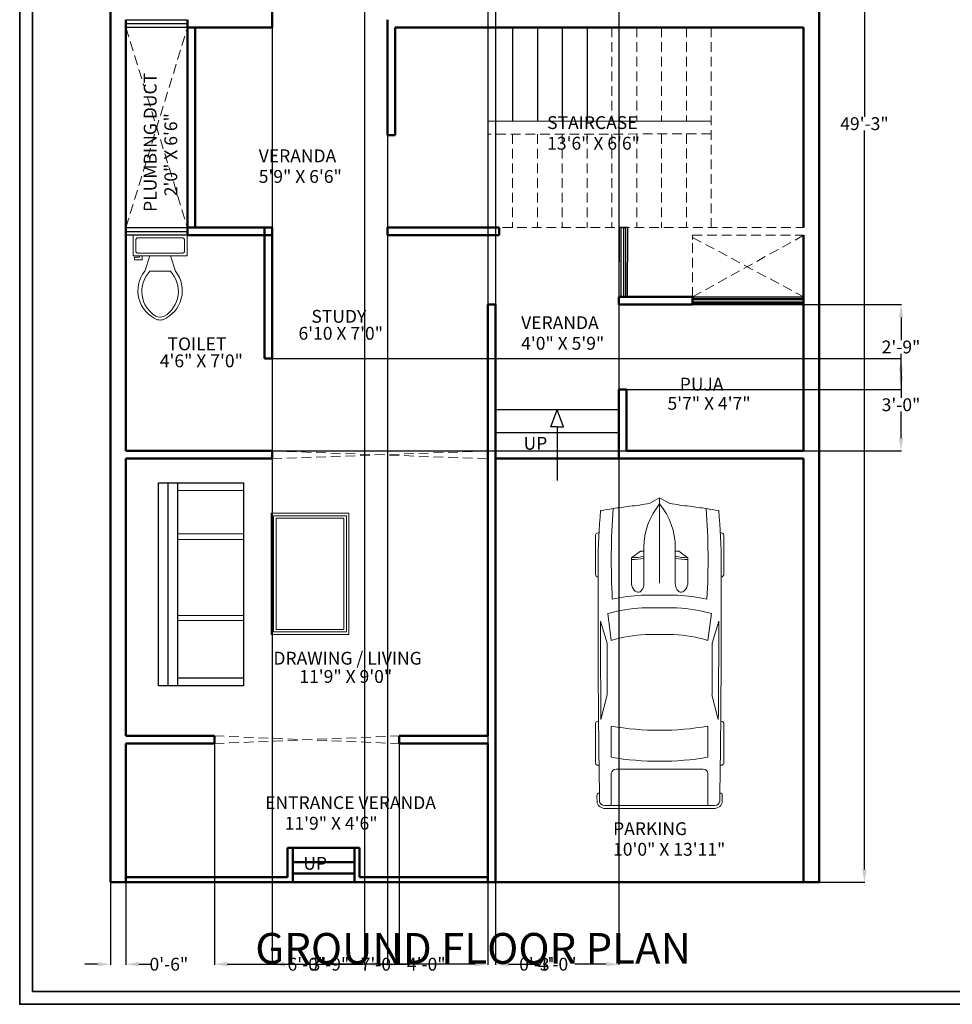
# Model space of a CAD drawing. Units: inches. Extents: x 396 to 1141, y -378 to 313.
# Tile 1 of 3: x 400 to 764, y -378 to 6. Entities that reach past the tile are written whole.
import ezdxf

# ---------------------------------------------------------------- set-up
doc = ezdxf.new("R2010")
doc.units = ezdxf.units.IN
doc.header["$MEASUREMENT"] = 0
doc.linetypes.add('DASHED', pattern=[19.05, 12.7, -6.35])
for name, color, linetype, lineweight in [('A-ANNO-DIMS', 2, 'Continuous', 18), ('A-ANNO-TTLB', 7, 'Continuous', 35), ('A-AREA-IDEN', 3, 'Continuous', 25), ('A-EQPM', 8, 'Continuous', 13), ('A-FLOR-FIXT', 150, 'Continuous', 18), ('A-FLOR-OVHD', 8, 'DASHED', 18), ('A-FLOR-STRS', 220, 'Continuous', 25), ('A-FLOR-STRS-OVHD', 220, 'DASHED', 18), ('A-FURN', 30, 'Continuous', 18), ('A-GLAZ', 4, 'Continuous', 25), ('A-WALL', 7, 'Continuous', 50)]:
    doc.layers.add(name, color=color, linetype=linetype, lineweight=lineweight)
doc.styles.get("Standard").update_dxf_attribs({"font": 'arial.ttf'})
doc.dimstyles.get("Standard").update_dxf_attribs({"dimtxt": 5, "dimasz": 5, "dimexe": 0.18, "dimexo": 0.0625, "dimgap": 0.09, "dimtad": 0, "dimtih": 1, "dimtoh": 1, "dimdec": 1, "dimzin": 0, "dimdsep": 46, "dimlunit": 4, "dimtxsty": 'Standard', "dimcen": 0.09, "dimadec": 0, "dimazin": 0, "dimtfac": 1, "dimtdec": 1, "dimtofl": 0, "dimtmove": 0, "dimatfit": 3, "dimfxl": 1, "dimtolj": 1, "dimtzin": 0, "dimarcsym": 0})

# ---------------------------------------------------------------- blocks, each defined once
blk = doc.blocks.new('*U6')
for p, q in [((9.5, -6), (9.5, -2)), ((-10, -8.5), (-8, -8.5)), ((-10, -9.5), (-10, -8.5)), ((-7, -9.5), (-10, -9.5)), ((-8, -8.5), (-8, -8)), ((-7, -8), (-7, -9.5)), ((-4, -8), (-6, -14)), ((4, -8), (6, -14)), ((4, -14), (-4, -14))]:
    blk.add_line(p, q)
blk.add_lwpolyline([(10.5, -8), (10.5, 0), (-10.5, 0), (-10.5, -8)], close=True)
for points in [[(-9.5, -2), (-9.5, -6)], [(8.5, -1), (-8.5, -1)], [(-8.5, -7), (8.5, -7)]]:
    blk.add_lwpolyline(points)
for centre, radius, start, end in [((-8.62, -1.88), 0.884, 81.8699, 188.1301), ((8.62, -1.88), 0.884, 351.8699, 98.1301), ((-8.62, -6.12), 0.884, 171.8699, 278.1301), ((8.62, -6.12), 0.884, 261.8699, 8.1301), ((3.52, -21.58), 12.17, 141.4691, 247.9714), ((4.2, -21.82), 11.33, 136.3677, 238.9468), ((-3.52, -21.58), 12.17, 292.0284, 38.5307), ((-4.2, -21.82), 11.33, 301.053, 43.6321), ((0, -27.88), 4, 245.7318, 294.2682), ((0, -29), 4, 254.8605, 285.1395)]:
    blk.add_arc(centre, radius, start, end)
blk = doc.blocks.new('*U8')
for p, q in [((21.1, 37.41), (21.1, 36.83)), ((46.55, 38.89), (22.35, 38.89)), ((47.8, 37.39), (47.8, 37.41)), ((87.99, 31.87), (74.76, 35.92)), ((135.45, 37.07), (135.45, 37.41)), ((136.7, 38.89), (160.9, 38.89)), ((162.15, 37.41), (162.15, 36.77)), ((70.03, 31.54), (86.41, 29.35)), ((134.31, 35.6), (119.29, 31.78)), ((186.47, -33.5), (186.47, 33.5)), ((188.4, -32.76), (188.4, 32.76)), ((138.42, 29.35), (157.25, 29.35)), ((164.52, 26.39), (164.52, -26.39)), ((186.47, 29.35), (167.01, 29.35)), ((32.27, 11.63), (36.13, 17.17)), ((36.13, 17.17), (50.94, 17.17)), ((3.27, 6.13), (0.1, 0.41)), ((29.77, 9.51), (51.68, 9.51)), ((32.12, 9.51), (32.12, 11.15)), ((58.92, -10.77), (58.92, 10.77)), ((66.55, -10.53), (66.55, 10.53)), ((82.74, 8.5), (82.74, -8.5)), ((186.47, -10.53), (186.47, 10.53)), ((0, 0), (51.68, 0)), ((0.1, -0.41), (3.27, -6.13)), ((29.77, -9.51), (51.68, -9.51)), ((32.12, -9.51), (32.12, -11.15)), ((32.27, -11.63), (36.13, -17.17)), ((36.13, -17.17), (50.94, -17.17)), ((86.41, -29.35), (70.03, -31.54)), ((157.25, -29.35), (138.42, -29.35)), ((167.01, -29.35), (186.47, -29.35)), ((87.99, -31.87), (74.76, -35.92)), ((134.31, -35.6), (119.29, -31.78)), ((21.1, -37.41), (21.1, -36.83)), ((46.55, -38.89), (22.35, -38.89)), ((47.8, -37.39), (47.8, -37.41)), ((135.45, -37.07), (135.45, -37.41)), ((136.7, -38.89), (160.9, -38.89)), ((162.15, -37.41), (162.15, -36.77))]:
    blk.add_line(p, q)
for centre, major_axis, ratio, start_param, end_param in [((266.03, -27.52), (0, 313.31), 0.842304, 1.367076, 1.39176), ((41.19, -490.86), (0, 528.23), 0.842304, 0.00281, 0.075598), ((22.35, 37.41), (0, -1.48), 0.842304, 3.141593, 4.712389), ((64.48, -10555.62), (0, 10593.03), 0.842304, -0.013397, 0.002797), ((46.55, 37.41), (0, 1.48), 0.842304, -1.570796, 0), ((64.48, -10555.62), (0, -10591.55), 0.842304, 3.133765, 3.140441), ((136.7, 37.41), (0, -1.48), 0.842304, 3.141593, 4.712389), ((160.9, 37.41), (0, 1.48), 0.842304, -1.570796, 0), ((180.63, 35.84), (0, 2.22), 0.842304, -0.013017, 1.249894), ((64.48, -10556.36), (0, 10595.31), 0.842304, -0.013397, -0.013017), ((183.98, 33.5), (0, -2.96), 0.842304, 1.570796, 3.128196), ((183.98, 32.76), (0, -5.25), 0.842304, 1.570796, 3.128196), ((135.29, 5.39), (0, 81.77), 0.842304, 1.245306, 1.50788), ((95.79, -3666.35), (0, -3698.24), 0.842304, 3.134049, 3.144098), ((259.18, -27.52), (0, -305.3), 0.842304, 4.528606, 4.561838), ((37.47, -593.96), (0, -623.33), 0.842304, 3.096046, 3.200911), ((134.4, 5.39), (0, -89.78), 0.842304, 4.449482, 4.652344), ((149.6, 2.8), (0, -79.58), 0.842304, 4.372215, 4.640744), ((17.08, 0), (0, 147.02), 0.842304, 4.511394, 4.913384), ((35.91, 0), (0, 147.02), 0.842304, 4.511394, 4.913384), ((167.01, 26.39), (0, 2.96), 0.842304, 0, 1.570796), ((-204.49, 52.4), (0, -250.96), 0.842304, 1.385369, 1.434372), ((13.04, 17.01), (0, 27.42), 0.842304, 4.435146, 4.718221), ((14.2, 17.01), (0, 27.42), 0.842304, 4.435146, 4.718221), ((50.79, 13.34), (6.34, -0.36), 0.603834, -1.395552, 1.581315), ((29.77, -46.66), (0, 56.17), 0.842304, 0, 0.590319), ((32.75, 11.15), (0, 0.74), 0.842304, 0.879714, 1.570796), ((0.62, 0), (0, -0.74), 0.842304, 4.131459, 5.293319), ((29.77, 46.66), (0, 56.17), 0.842304, 2.551274, 3.141593), ((-204.49, -52.4), (0, 250.96), 0.842304, -1.434372, -1.385369), ((32.75, -11.15), (0, -0.74), 0.842304, 4.712389, 5.403472), ((13.04, -17.01), (0, -27.42), 0.842304, 1.564964, 1.848039), ((14.2, -17.01), (0, -27.42), 0.842304, 1.564964, 1.848039), ((134.4, -5.39), (0, -89.78), 0.842304, -1.510751, -1.307889), ((135.29, -5.39), (0, -81.77), 0.842304, -1.50788, -1.245306), ((149.6, -2.8), (0, -79.58), 0.842304, -1.499151, -1.230623), ((259.18, 27.52), (0, 305.3), 0.842304, 1.721348, 1.754579), ((266.03, 27.52), (0, 313.31), 0.842304, 1.749832, 1.774517), ((37.47, 593.96), (0, -623.33), 0.842304, -0.059319, 0.045547), ((167.01, -26.39), (0, -2.96), 0.842304, 4.712389, 6.283185), ((64.48, 10555.62), (0, -10591.55), 0.842304, 0.001152, 0.007828), ((95.79, 3666.35), (0, -3698.24), 0.842304, -0.002505, 0.007544), ((183.98, -33.5), (0, 2.96), 0.842304, 3.15499, 4.712389), ((183.98, -32.76), (0, -5.25), 0.842304, 0.013397, 1.570796), ((41.19, 490.86), (0, -528.23), 0.842304, -0.075598, -0.00281), ((22.35, -37.41), (0, 1.48), 0.842304, 1.570796, 3.141593), ((64.48, 10555.62), (0, 10593.03), 0.842304, 3.138796, 3.15499), ((46.55, -37.41), (0, -1.48), 0.842304, 0, 1.570796), ((136.7, -37.41), (0, -1.48), 0.842304, -1.570796, 0), ((160.9, -37.41), (0, 1.48), 0.842304, 3.141593, 4.712389), ((180.63, -35.84), (0, -2.22), 0.842304, -1.249894, 0.013017), ((64.48, 10556.36), (0, 10595.31), 0.842304, 3.15461, 3.15499)]:
    blk.add_ellipse(centre, major_axis=major_axis, ratio=ratio, start_param=start_param, end_param=end_param)
at = {"extrusion": (0, 0, -1)}
blk.add_ellipse((50.79, -13.34), major_axis=(6.34, 0.36), ratio=0.603834, start_param=-1.395552, end_param=1.581315, dxfattribs=at)
blk = doc.blocks.new('*D10')
at = {"layer": 'A-ANNO-DIMS', "color": 0, "lineweight": -2, "ltscale": 0.3, "transparency": 16777216}
for p, q in [((711.68, 260.95), (729.49, 260.95)), ((729.31, 255.95), (729.31, -31.9)), ((729.31, -325.05), (729.31, -37.19)), ((711.68, -330.05), (729.49, -330.05))]:
    blk.add_line(p, q, dxfattribs=at)
at = {"layer": 'A-ANNO-DIMS', "color": 0, "ltscale": 0.3, "transparency": 16777216}
for points in [[(728.47, 255.95), (730.14, 255.95), (729.31, 260.95)], [(728.47, -325.05), (730.14, -325.05), (729.31, -330.05)]]:
    blk.add_solid(points, dxfattribs=at)
at = {"layer": 'Defpoints', "color": 0, "ltscale": 0.3, "transparency": 16777216}
for p in [(711.61, 260.95), (711.61, -330.05), (729.31, -330.05)]:
    blk.add_point(p, dxfattribs=at)
at = {"layer": 'A-ANNO-DIMS', "color": 0, "ltscale": 0.3, "transparency": 16777216, "insert": (729.31, -34.55), "char_height": 5, "attachment_point": 5}
blk.add_mtext('\\A1;49\'-3"', dxfattribs=at)
blk = doc.blocks.new('WIN-DUCT-700')
at = {"ltscale": 0.3}
blk.add_line((441.61, 4.45), (465.61, 4.45), dxfattribs=at)
blk.add_lwpolyline([(441.61, 5.95), (465.61, 5.95), (465.61, 2.95), (441.61, 2.95)], close=True, dxfattribs=at)
blk = doc.blocks.new('*D31')
at = {"layer": 'A-ANNO-DIMS', "color": 0, "lineweight": -2, "ltscale": 0.3, "transparency": 16777216}
for p, q in [((441.61, -328.11), (441.61, -362.18)), ((435.61, -330.11), (435.61, -362.18)), ((430.61, -362), (425.61, -362)), ((446.61, -362), (451.61, -362))]:
    blk.add_line(p, q, dxfattribs=at)
at = {"layer": 'A-ANNO-DIMS', "color": 0, "ltscale": 0.3, "transparency": 16777216}
for points in [[(430.61, -361.16), (430.61, -362.83), (435.61, -362)], [(446.61, -361.16), (446.61, -362.83), (441.61, -362)]]:
    blk.add_solid(points, dxfattribs=at)
at = {"layer": 'Defpoints', "color": 0, "ltscale": 0.3, "transparency": 16777216}
for p in [(441.61, -328.05), (435.61, -330.05), (441.61, -362)]:
    blk.add_point(p, dxfattribs=at)
at = {"layer": 'A-ANNO-DIMS', "color": 0, "ltscale": 0.3, "transparency": 16777216, "insert": (458.35, -362), "char_height": 5, "attachment_point": 5}
blk.add_mtext('\\A1;0\'-6"', dxfattribs=at)
blk = doc.blocks.new('*D32')
at = {"layer": 'A-ANNO-DIMS', "color": 0, "lineweight": -2, "ltscale": 0.3, "transparency": 16777216}
for p, q in [((582.61, 125.89), (582.61, -362.18)), ((585.61, 125.89), (585.61, -362.18)), ((577.61, -362), (572.61, -362)), ((590.61, -362), (595.61, -362))]:
    blk.add_line(p, q, dxfattribs=at)
at = {"layer": 'A-ANNO-DIMS', "color": 0, "ltscale": 0.3, "transparency": 16777216}
for points in [[(577.61, -361.16), (577.61, -362.83), (582.61, -362)], [(590.61, -361.16), (590.61, -362.83), (585.61, -362)]]:
    blk.add_solid(points, dxfattribs=at)
at = {"layer": 'Defpoints', "color": 0, "ltscale": 0.3, "transparency": 16777216}
for p in [(582.61, 125.95), (585.61, 125.95), (585.61, -362)]:
    blk.add_point(p, dxfattribs=at)
at = {"layer": 'A-ANNO-DIMS', "color": 0, "ltscale": 0.3, "transparency": 16777216, "insert": (602.35, -362), "char_height": 5, "attachment_point": 5}
blk.add_mtext('\\A1;0\'-3"', dxfattribs=at)
blk = doc.blocks.new('*D33')
at = {"layer": 'A-ANNO-DIMS', "color": 0, "lineweight": -2, "ltscale": 0.3, "transparency": 16777216}
for p, q in [((534.61, 125.89), (534.61, -362.18)), ((582.61, 125.89), (582.61, -362.18)), ((539.61, -362), (551.78, -362)), ((577.61, -362), (565.45, -362))]:
    blk.add_line(p, q, dxfattribs=at)
at = {"layer": 'A-ANNO-DIMS', "color": 0, "ltscale": 0.3, "transparency": 16777216}
for points in [[(539.61, -361.16), (539.61, -362.83), (534.61, -362)], [(577.61, -361.16), (577.61, -362.83), (582.61, -362)]]:
    blk.add_solid(points, dxfattribs=at)
at = {"layer": 'Defpoints', "color": 0, "ltscale": 0.3, "transparency": 16777216}
for p in [(534.61, 125.95), (582.61, 125.95), (582.61, -362)]:
    blk.add_point(p, dxfattribs=at)
at = {"layer": 'A-ANNO-DIMS', "color": 0, "ltscale": 0.3, "transparency": 16777216, "insert": (558.61, -362), "char_height": 5, "attachment_point": 5}
blk.add_mtext('\\A1;4\'-0"', dxfattribs=at)
blk = doc.blocks.new('*D34')
at = {"layer": 'A-ANNO-DIMS', "color": 0, "lineweight": -2, "ltscale": 0.3, "transparency": 16777216}
for p, q in [((585.61, 125.89), (585.61, -362.18)), ((633.61, 125.89), (633.61, -362.18)), ((590.61, -362), (602.78, -362)), ((628.61, -362), (616.45, -362))]:
    blk.add_line(p, q, dxfattribs=at)
at = {"layer": 'A-ANNO-DIMS', "color": 0, "ltscale": 0.3, "transparency": 16777216}
for points in [[(590.61, -361.16), (590.61, -362.83), (585.61, -362)], [(628.61, -361.16), (628.61, -362.83), (633.61, -362)]]:
    blk.add_solid(points, dxfattribs=at)
at = {"layer": 'Defpoints', "color": 0, "ltscale": 0.3, "transparency": 16777216}
for p in [(585.61, 125.95), (633.61, 125.95), (633.61, -362)]:
    blk.add_point(p, dxfattribs=at)
at = {"layer": 'A-ANNO-DIMS', "color": 0, "ltscale": 0.3, "transparency": 16777216, "insert": (609.61, -362), "char_height": 5, "attachment_point": 5}
blk.add_mtext('\\A1;4\'-0"', dxfattribs=at)
blk = doc.blocks.new('*D35')
at = {"layer": 'A-ANNO-DIMS', "color": 0, "lineweight": -2, "ltscale": 0.3, "transparency": 16777216}
for p, q in [((543.55, 5.89), (543.55, -362.18)), ((498.61, 2.89), (498.61, -362.18)), ((503.61, -362), (514.35, -362)), ((538.55, -362), (527.82, -362))]:
    blk.add_line(p, q, dxfattribs=at)
at = {"layer": 'A-ANNO-DIMS', "color": 0, "ltscale": 0.3, "transparency": 16777216}
for points in [[(503.61, -361.16), (503.61, -362.83), (498.61, -362)], [(538.55, -361.16), (538.55, -362.83), (543.55, -362)]]:
    blk.add_solid(points, dxfattribs=at)
at = {"layer": 'Defpoints', "color": 0, "ltscale": 0.3, "transparency": 16777216}
for p in [(543.55, 5.95), (498.61, 2.95), (543.55, -362)]:
    blk.add_point(p, dxfattribs=at)
at = {"layer": 'A-ANNO-DIMS', "color": 0, "ltscale": 0.3, "transparency": 16777216, "insert": (521.08, -362), "char_height": 5, "attachment_point": 5}
blk.add_mtext('\\A1;3\'-9"', dxfattribs=at)
blk = doc.blocks.new('*D36')
at = {"layer": 'A-ANNO-DIMS', "color": 0, "lineweight": -2, "ltscale": 0.3, "transparency": 16777216}
for p, q in [((498.68, -126.05), (743.74, -126.05)), ((743.56, -131.05), (743.56, -141.4)), ((743.56, -157.05), (743.56, -146.69)), ((498.68, -162.05), (743.74, -162.05))]:
    blk.add_line(p, q, dxfattribs=at)
at = {"layer": 'A-ANNO-DIMS', "color": 0, "ltscale": 0.3, "transparency": 16777216}
for points in [[(742.73, -131.05), (744.4, -131.05), (743.56, -126.05)], [(742.73, -157.05), (744.4, -157.05), (743.56, -162.05)]]:
    blk.add_solid(points, dxfattribs=at)
at = {"layer": 'Defpoints', "color": 0, "ltscale": 0.3, "transparency": 16777216}
for p in [(498.61, -126.05), (498.61, -162.05), (743.56, -162.05)]:
    blk.add_point(p, dxfattribs=at)
at = {"layer": 'A-ANNO-DIMS', "color": 0, "ltscale": 0.3, "transparency": 16777216, "insert": (743.56, -144.05), "char_height": 5, "attachment_point": 5}
blk.add_mtext('\\A1;3\'-0"', dxfattribs=at)
blk = doc.blocks.new('*D37')
at = {"layer": 'A-ANNO-DIMS', "color": 0, "lineweight": -2, "ltscale": 0.3, "transparency": 16777216}
for p, q in [((498.61, -162.11), (498.61, -362.18)), ((582.61, -162.11), (582.61, -362.18)), ((503.61, -362), (533.9, -362)), ((577.61, -362), (547.33, -362))]:
    blk.add_line(p, q, dxfattribs=at)
at = {"layer": 'A-ANNO-DIMS', "color": 0, "ltscale": 0.3, "transparency": 16777216}
for points in [[(503.61, -361.16), (503.61, -362.83), (498.61, -362)], [(577.61, -361.16), (577.61, -362.83), (582.61, -362)]]:
    blk.add_solid(points, dxfattribs=at)
at = {"layer": 'Defpoints', "color": 0, "ltscale": 0.3, "transparency": 16777216}
for p in [(498.61, -162.05), (582.61, -162.05), (582.61, -362)]:
    blk.add_point(p, dxfattribs=at)
at = {"layer": 'A-ANNO-DIMS', "color": 0, "ltscale": 0.3, "transparency": 16777216, "insert": (540.61, -362), "char_height": 5, "attachment_point": 5}
blk.add_mtext('\\A1;7\'-0"', dxfattribs=at)
blk = doc.blocks.new('*D38')
at = {"layer": 'A-ANNO-DIMS', "color": 0, "lineweight": -2, "ltscale": 0.3, "transparency": 16777216}
for p, q in [((476.11, -273.11), (476.11, -362.18)), ((548.11, -273.11), (548.11, -362.18)), ((481.11, -362), (505.36, -362)), ((543.11, -362), (518.86, -362))]:
    blk.add_line(p, q, dxfattribs=at)
at = {"layer": 'A-ANNO-DIMS', "color": 0, "ltscale": 0.3, "transparency": 16777216}
for points in [[(481.11, -361.16), (481.11, -362.83), (476.11, -362)], [(543.11, -361.16), (543.11, -362.83), (548.11, -362)]]:
    blk.add_solid(points, dxfattribs=at)
at = {"layer": 'Defpoints', "color": 0, "ltscale": 0.3, "transparency": 16777216}
for p in [(476.11, -273.05), (548.11, -273.05), (548.11, -362)]:
    blk.add_point(p, dxfattribs=at)
at = {"layer": 'A-ANNO-DIMS', "color": 0, "ltscale": 0.3, "transparency": 16777216, "insert": (512.11, -362), "char_height": 5, "attachment_point": 5}
blk.add_mtext('\\A1;6\'-0"', dxfattribs=at)
blk = doc.blocks.new('*D39')
at = {"layer": 'A-ANNO-DIMS', "color": 0, "lineweight": -2, "ltscale": 0.3, "transparency": 16777216}
for p, q in [((633.68, -105.05), (743.74, -105.05)), ((743.56, -110.05), (743.56, -118.9)), ((743.56, -133.05), (743.56, -124.19)), ((633.68, -138.05), (743.74, -138.05))]:
    blk.add_line(p, q, dxfattribs=at)
at = {"layer": 'A-ANNO-DIMS', "color": 0, "ltscale": 0.3, "transparency": 16777216}
for points in [[(742.73, -110.05), (744.4, -110.05), (743.56, -105.05)], [(742.73, -133.05), (744.4, -133.05), (743.56, -138.05)]]:
    blk.add_solid(points, dxfattribs=at)
at = {"layer": 'Defpoints', "color": 0, "ltscale": 0.3, "transparency": 16777216}
for p in [(633.61, -105.05), (633.61, -138.05), (743.56, -138.05)]:
    blk.add_point(p, dxfattribs=at)
at = {"layer": 'A-ANNO-DIMS', "color": 0, "ltscale": 0.3, "transparency": 16777216, "insert": (743.56, -121.55), "char_height": 5, "attachment_point": 5}
blk.add_mtext('\\A1;2\'-9"', dxfattribs=at)

msp = doc.modelspace()

# ---------------------------------------------------------------- linework, layer by layer
at = {"layer": 'A-ANNO-TTLB', "ltscale": 0.3}
for points in [[(400.24, 313.19), (1105.01, 313.19), (1105.01, -377.62), (400.24, -377.62)], [(405.24, 308.19), (1100.01, 308.19), (1100.01, -372.62), (405.24, -372.62)]]:
    msp.add_lwpolyline(points, close=True, dxfattribs=at)
at = {"layer": 'A-FLOR-OVHD', "ltscale": 0.3}
for p, q in [((441.61, 2.95), (465.61, -75.05)), ((441.61, -75.05), (465.61, 2.95)), ((662.34, -79.69), (662.34, -78.05)), ((662.34, -78.05), (705.61, -78.05)), ((662.34, -102.05), (705.61, -78.05)), ((662.34, -78.87), (705.61, -102.05)), ((662.34, -102.05), (662.34, -79.69)), ((498.61, -165.05), (582.61, -162.05)), ((498.61, -162.05), (582.61, -165.05)), ((476.11, -273.05), (548.11, -276.05)), ((476.11, -276.05), (548.11, -273.05))]:
    msp.add_line(p, q, dxfattribs=at)
at = {"layer": 'A-FLOR-STRS', "ltscale": 0.3}
for p, q in [((582.55, 2.85), (582.55, -33.65)), ((592.22, 2.86), (592.22, -33.64)), ((601.9, 2.87), (601.9, -33.63)), ((611.57, 2.88), (611.57, -33.62)), ((621.24, 2.9), (621.24, -33.6)), ((669.61, -33.54), (582.55, -33.65)), ((669.61, -38.93), (669.61, -38.9)), ((582.55, -75.05), (582.55, -75.15)), ((633.61, -145.98), (585.61, -145.98)), ((607.1, -152.67), (609.61, -145.98)), ((612.13, -152.67), (609.61, -145.98)), ((609.61, -152.67), (607.1, -152.67)), ((609.61, -152.67), (609.61, -173.51)), ((609.61, -152.67), (612.13, -152.67)), ((633.61, -155.05), (585.61, -155.05))]:
    msp.add_line(p, q, dxfattribs=at)
at = {"layer": 'A-FLOR-STRS-OVHD', "ltscale": 0.3}
for p, q in [((630.92, 2.91), (630.92, -33.59)), ((640.59, 2.92), (640.59, -33.58)), ((650.27, 2.93), (650.27, -33.57)), ((659.94, 2.95), (659.94, -33.55)), ((669.61, 2.96), (669.61, -75.04)), ((669.62, -38.54), (582.55, -38.65)), ((582.55, -38.65), (582.55, -75.05)), ((592.22, -38.64), (592.22, -75.14)), ((601.9, -38.63), (601.9, -75.13)), ((611.57, -38.62), (611.57, -75.12)), ((621.24, -38.6), (621.24, -75.1)), ((630.92, -38.59), (630.92, -75.09)), ((640.59, -38.58), (640.59, -75.08)), ((650.27, -38.57), (650.27, -75.07)), ((659.94, -38.55), (659.94, -75.05)), ((582.55, -75.05), (705.61, -75.05))]:
    msp.add_line(p, q, dxfattribs=at)
at = {"layer": 'A-FURN', "ltscale": 0.3}
for p, q in [((461.71, -177.47), (487.38, -177.47)), ((461.71, -194.35), (487.38, -194.35)), ((461.71, -196.5), (487.38, -196.5)), ((461.71, -226.11), (487.38, -226.11)), ((461.71, -228.12), (487.38, -228.12))]:
    msp.add_line(p, q, dxfattribs=at)
for points in [[(498.15, -186.28), (528.49, -186.28), (528.49, -233.57), (498.15, -233.57)], [(499.15, -187.28), (527.49, -187.28), (527.49, -232.57), (499.15, -232.57)], [(500.15, -188.28), (526.49, -188.28), (526.49, -231.57), (500.15, -231.57)], [(500.15, -188.28), (526.49, -188.28), (526.49, -231.57), (500.15, -231.57)], [(500.15, -188.28), (526.49, -188.28), (526.49, -231.57), (500.15, -231.57)]]:
    msp.add_lwpolyline(points, close=True, dxfattribs=at)
at = {"layer": 'A-GLAZ', "ltscale": 0.3}
for p, q in [((635.43, -75.05), (635.43, -102.05)), ((457.97, -174.42), (457.97, -253.57)), ((461.71, -174.42), (461.71, -253.57)), ((487.38, -250.57), (461.71, -250.57))]:
    msp.add_line(p, q, dxfattribs=at)
for points in [[(633.61, -102.05), (637.03, -102.05), (637.13, -75.05), (633.72, -75.05)], [(634.59, -75.05), (636.26, -75.05), (636.26, -102.05), (634.59, -102.05)], [(662.34, -102.05), (705.61, -102.05), (705.61, -105.05), (662.34, -105.05)], [(662.34, -102.68), (705.61, -102.68), (705.61, -104.58), (662.34, -104.58)], [(662.34, -103.05), (705.61, -103.05), (705.61, -104.13), (662.34, -104.13)], [(454.36, -174.42), (487.38, -174.42), (487.38, -253.57), (454.36, -253.57)]]:
    msp.add_lwpolyline(points, close=True, dxfattribs=at)
at = {"layer": 'A-WALL'}
for p, q in [((435.61, 260.95), (435.61, -330.05)), ((711.61, 260.95), (711.61, -330.05)), ((498.61, 125.95), (498.61, 2.95)), ((441.61, 5.95), (441.61, 2.95)), ((465.61, 2.95), (465.61, 5.95)), ((543.55, 5.95), (543.55, -39.05)), ((441.61, 2.95), (441.61, -75.05)), ((465.61, 2.95), (465.61, -78.05)), ((498.61, 2.95), (465.61, 2.95)), ((468.61, 2.95), (468.61, -75.05)), ((705.61, 2.95), (546.55, 2.95)), ((546.55, 2.95), (546.55, -39.05)), ((705.61, 2.95), (705.61, -75.05)), ((441.61, -78.05), (441.61, -75.05)), ((498.61, -75.05), (465.61, -75.05)), ((495.61, -75.05), (495.61, -126.05)), ((498.61, -75.05), (498.61, -126.05)), ((586.96, -75.05), (543.55, -75.05)), ((441.61, -78.05), (441.61, -162.05)), ((498.61, -78.05), (465.61, -78.05)), ((586.96, -78.05), (543.55, -78.05)), ((705.61, -78.05), (705.61, -162.05)), ((662.34, -102.05), (633.61, -102.05)), ((582.61, -105.05), (582.61, -273.05)), ((585.61, -105.05), (582.61, -105.05)), ((585.61, -105.05), (585.61, -330.05)), ((662.34, -105.05), (633.61, -105.05)), ((498.61, -126.05), (495.61, -126.05)), ((498.61, -162.05), (441.61, -162.05)), ((498.61, -162.05), (498.61, -165.05)), ((705.61, -162.05), (636.61, -162.05)), ((441.61, -165.05), (441.61, -273.05)), ((498.61, -165.05), (441.61, -165.05)), ((705.61, -165.05), (633.61, -165.05)), ((705.61, -165.05), (705.61, -330.05)), ((476.11, -273.05), (441.61, -273.05)), ((441.61, -276.05), (441.61, -330.05)), ((476.11, -276.05), (441.61, -276.05)), ((476.11, -276.05), (476.11, -273.05)), ((548.11, -276.05), (548.11, -273.05)), ((582.61, -273.05), (548.11, -273.05)), ((582.61, -276.05), (548.11, -276.05)), ((582.61, -276.05), (582.61, -330.05))]:
    msp.add_line(p, q, dxfattribs=at)
at = {"layer": 'A-WALL', "ltscale": 0.3}
for p, q in [((546.55, -39.05), (543.55, -39.05)), ((543.55, -78.05), (543.55, -75.05)), ((586.96, -75.05), (586.96, -78.05)), ((633.61, -105.05), (633.61, -102.05)), ((662.34, -102.05), (662.34, -105.05)), ((633.61, -162.05), (633.61, -138.05)), ((633.61, -138.05), (636.61, -138.05)), ((636.61, -162.05), (636.61, -138.05)), ((633.61, -162.05), (633.61, -165.05)), ((633.61, -165.05), (585.61, -165.05)), ((504.62, -316.6), (504.62, -328.05)), ((504.62, -316.6), (506.62, -316.6)), ((506.62, -316.6), (506.62, -330.05)), ((506.62, -316.6), (530.62, -316.6)), ((530.62, -316.6), (530.62, -330.05)), ((530.62, -316.6), (532.62, -316.6)), ((532.62, -316.6), (532.62, -328.05)), ((506.62, -322.29), (530.62, -322.29)), ((504.62, -328.05), (441.61, -328.05)), ((506.62, -326.61), (530.62, -326.61)), ((532.62, -328.05), (582.61, -328.05)), ((435.61, -330.05), (441.61, -330.05)), ((441.61, -330.05), (506.62, -330.05)), ((506.62, -330.05), (530.62, -330.05)), ((530.62, -330.05), (582.61, -330.05)), ((585.61, -330.05), (582.61, -330.05)), ((585.61, -330.05), (705.61, -330.05)), ((705.61, -330.05), (711.61, -330.05))]:
    msp.add_line(p, q, dxfattribs=at)

# ---------------------------------------------------------------- block references
at = {"layer": 'A-EQPM', "xscale": 0.641757873664314, "yscale": 0.641757873664314, "zscale": 0.641757873664314, "rotation": 270}
msp.add_blockref('*U8', (649.53, -180.44), dxfattribs=at)
at = {"layer": 'A-FLOR-FIXT'}
msp.add_blockref('*U6', (454.94, -78.05), dxfattribs=at)
at = {"layer": 'A-GLAZ'}
for p in [(0, 0), (0, -81)]:
    msp.add_blockref('WIN-DUCT-700', p, dxfattribs=at)

# ---------------------------------------------------------------- texts
at = {"layer": 'A-AREA-IDEN', "ltscale": 0.3}
for s, p in [('PLUMBING DUCT', (453.58, -68.93)), ('    2\'0" X 6\'6"', (461.61, -68.93))]:
    msp.add_text(s, height=5, rotation=90, dxfattribs=at).set_placement(p)
for s, height, p in [('STAIRCASE', 5, (605.71, -36.64)), ('13\'6" X 6\'6"', 5, (605.71, -44.68)), ('VERANDA', 5, (493.36, -49.59)), ('5\'9" X 6\'6"', 5, (493.36, -57.62)), ('STUDY', 5, (513.87, -112.11)), ('VERANDA', 5, (595.59, -114.58)), ('6\'10 X 7\'0"', 5, (508.85, -118.72)), ('TOILET', 5, (457.84, -122.84)), ('4\'0" X 5\'9"', 5, (595.59, -122.61)), ('4\'6" X 7\'0"', 5, (454.82, -129.45)), ('PUJA ', 5, (657.37, -138.54)), ('5\'7" X 4\'7"', 5, (652.59, -146.02)), ('UP', 5, (596.52, -161.57)), ('DRAWING / LIVING', 5, (499.08, -245.3)), ('11\'9" X 9\'0"', 5, (509.19, -252.41)), ('ENTRANCE VERANDA', 5, (495.85, -301.56)), ('     11\'9" X 4\'6"', 5, (495.85, -309.59)), ('PARKING', 5, (631.39, -311.71)), ('10\'0" X 13\'11"', 5, (631.39, -319.74)), ('UP', 5, (510.71, -325.21)), ('GROUND FLOOR PLAN', 12, (492.02, -361.84))]:
    msp.add_text(s, height=height, dxfattribs=at).set_placement(p)

# ---------------------------------------------------------------- dimensions: what is measured, and where the dimension line sits
at = {"layer": 'A-ANNO-DIMS', "ltscale": 0.3}
for base, p1, p2, override, picture, middle in [((729.31, -330.05), (711.61, 260.95), (711.61, -330.05), {"dimclrd": 0, "dimclre": 0, "dimclrt": 0}, '*D10', (729.31, -34.55)), ((743.56, -138.05), (633.61, -105.05), (633.61, -138.05), {"dimdec": 1, "dimlfac": 1, "dimrnd": 0, "dimzin": 1, "dimdsep": 46, "dimlunit": 4, "dimfrac": 2}, '*D39', (743.56, -121.55)), ((743.56, -162.05), (498.61, -126.05), (498.61, -162.05), {"dimdec": 1, "dimlfac": 1, "dimrnd": 0, "dimzin": 1, "dimdsep": 46, "dimlunit": 4, "dimfrac": 2}, '*D36', (743.56, -144.05))]:
    dim = msp.add_linear_dim(base=base, p1=p1, p2=p2, angle=90, dimstyle='Standard', override=override, dxfattribs=at)
    dim.commit()
    dim.dimension.update_dxf_attribs({"geometry": picture, "text_midpoint": middle})
for base, p1, p2, picture, middle in [((582.61, -362), (534.61, 125.95), (582.61, 125.95), '*D33', (558.61, -362)), ((585.61, -362), (582.61, 125.95), (585.61, 125.95), '*D32', (602.35, -362)), ((633.61, -362), (585.61, 125.95), (633.61, 125.95), '*D34', (609.61, -362)), ((543.55, -362), (498.61, 2.95), (543.55, 5.95), '*D35', (521.08, -362)), ((582.61, -362), (498.61, -162.05), (582.61, -162.05), '*D37', (540.61, -362)), ((548.11, -362), (476.11, -273.05), (548.11, -273.05), '*D38', (512.11, -362)), ((441.61, -362), (435.61, -330.05), (441.61, -328.05), '*D31', (458.35, -362))]:
    dim = msp.add_linear_dim(base=base, p1=p1, p2=p2, dimstyle='Standard', override={"dimdec": 1, "dimlfac": 1, "dimrnd": 0, "dimzin": 1, "dimdsep": 46, "dimlunit": 4, "dimfrac": 2}, dxfattribs=at)
    dim.commit()
    dim.dimension.update_dxf_attribs({"geometry": picture, "text_midpoint": middle})

doc.saveas('drawing.dxf')
